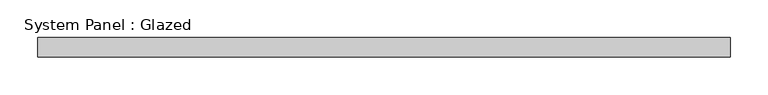
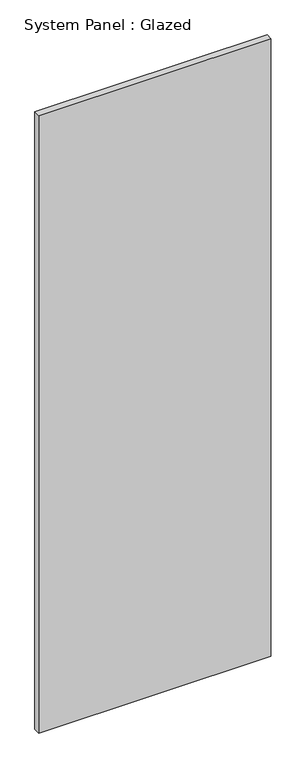
"""IFC4 building model written with IfcOpenShell, lengths in millimetres: plate geometry, System Panel : Glazed."""

from ifc_helpers import new_model, si_unit, origin, origin_with_axes, place, context, project, spatial, polyline, outline, extrude, source, transform, mapped, element, save


def system_panel_glazed_9aa1dd94(model_context):
    return source(origin(), model_context, "Body", "SweptSolid", [
        extrude(outline(polyline([(457.2, 19.05), (-457.2, 19.05), (-457.2, 44.45), (457.2, 44.45), (457.2, 19.05)])), origin_with_axes(), (0.0, 0.0, 1.0), 2570.5950276),
    ])


if __name__ == "__main__":
    model = new_model("IFC4")
    model_context = context("Model", 3, world=origin())
    ifc_project = project(units=[si_unit("LENGTHUNIT", "METRE", prefix="MILLI")], contexts=[model_context])
    site = spatial("IfcSite", under=ifc_project)
    building = spatial("IfcBuilding", under=site)
    placement = place(None, origin())
    system_panel_glazed_shape = system_panel_glazed_9aa1dd94(model_context)
    element("IfcPlate", 1, ObjectType="System Panel : Glazed", at=placement, inside=building, context=model_context, shape_type="MappedRepresentation", body=[
        mapped(system_panel_glazed_shape, transform((0.0, 0.0, 0.0), x_axis=(1.0, 0.0, 0.0), y_axis=(0.0, 1.0, 0.0), z_axis=(0.0, 0.0, 1.0))),
    ])
    save(model, "model.ifc")

# Revit data of these elements
# Type "System Panel : Glazed"
#   Construction Type Id = "GSP4R"
#   Analytic Construction = "1/8 in Pilkington single glazing"
#   Visual Light Transmittance = 0.9
#   Solar Heat Gain Coefficient = 0.86
#   Heat Transfer Coefficient (U) = 1.18115 BTU/(h·ft²·°F)
#   Define Thermal Properties by = 1
# Element 1 (IfcPlate, "System Panel : Glazed")
#   Materials on its faces: "Glass"
# Materials
#   "Glass": class "Glass", colour RGB 0 128 192, transparency 0.75, Description = "Soda Lime Glass", Cost = 0
